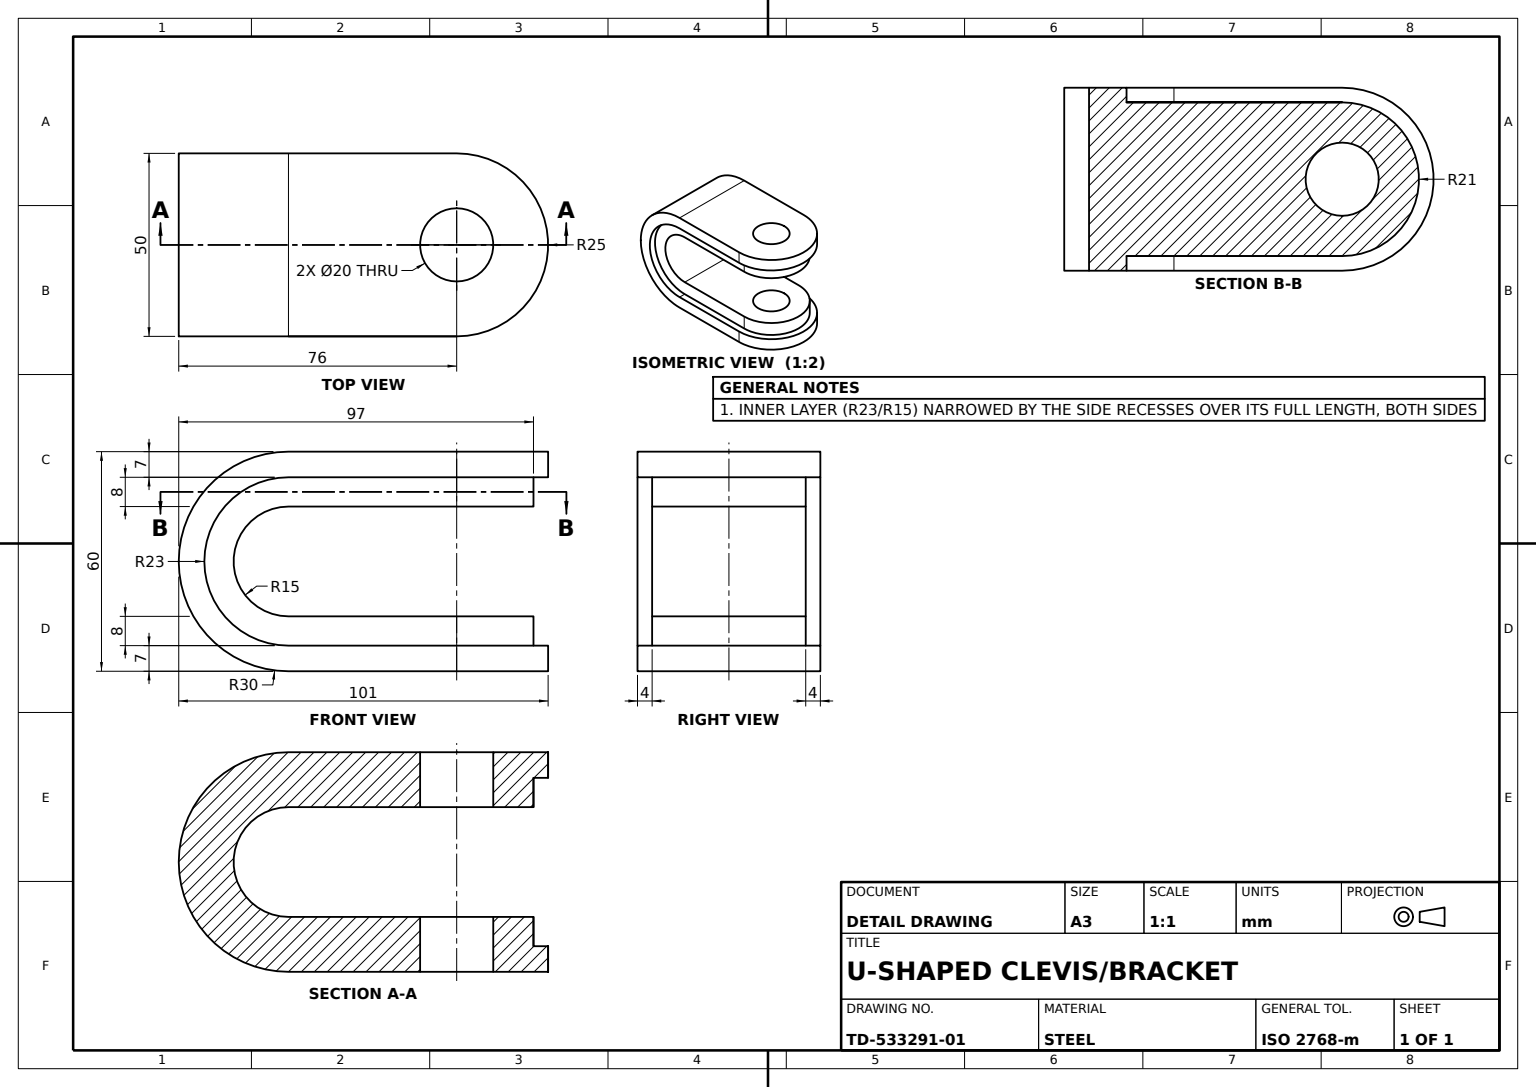
from build123d import *

# Parameters (mm, degrees)
U_FORK_BASE_DEPTH   = 50
U_START             = -50
U_WRAP_LAYER_DEPTH  = 50
WRAP_START          = -4
WRAP_RECESS_1_DEPTH = 4
WRAP_RECESS_2_DEPTH = 4
ARM_PAD_1_DEPTH     = 8
ARM_PAD_2_DEPTH     = 8
ARM_START           = -8
ARM_PAD_3_DEPTH     = 8
ARM_PAD_4_DEPTH     = 8
ARM_PAD_5_DEPTH     = 8
PIN_HOLE_SKETCH_R   = 10
PIN_HOLE_DEPTH      = 70
FACE_RELIEF_1_DEPTH = 1
FACE_START          = -1
FACE_RELIEF_2_DEPTH = 1


with BuildPart() as part:
    # U Fork Profile Sketch → U Fork Base (new body)
    with BuildSketch(Plane.XY):
        with BuildLine():
            ThreePointArc((0, 53), (-23, 30), (0, 7))
            Line((0, 7), (46, 7))
            Line((46, 7), (46, 0))
            Line((46, 0), (0, 0))
            ThreePointArc((0, 0), (-30, 30), (0, 60))
            Line((0, 60), (46, 60))
            Line((46, 60), (46, 53))
            Line((46, 53), (0, 53))
        make_face()
    extrude(amount=U_FORK_BASE_DEPTH)

    # U Wrap Layer Sketch → U Wrap Layer (add)
    with BuildSketch(Plane.XY.offset(50).offset(U_START)):
        with BuildLine():
            Line((0, 53), (46, 53))
            Line((46, 53), (46, 45))
            Line((46, 45), (0, 45))
            ThreePointArc((0, 45), (-15, 30), (0, 15))
            Line((0, 15), (46, 15))
            Line((46, 15), (46, 7))
            Line((46, 7), (0, 7))
            ThreePointArc((0, 7), (-23, 30), (0, 53))
        make_face()
    extrude(amount=U_WRAP_LAYER_DEPTH)

    # Wrap Recess 1 Sketch → Wrap Recess 1 (cut)
    with BuildSketch(Plane.XY.offset(50).offset(WRAP_START)):
        with BuildLine():
            Line((0, 45), (46, 45))
            Line((46, 45), (46, 53))
            Line((46, 53), (0, 53))
            ThreePointArc((0, 53), (-23, 30), (0, 7))
            Line((0, 7), (46, 7))
            Line((46, 7), (46, 15))
            Line((46, 15), (0, 15))
            ThreePointArc((0, 15), (-15, 30), (0, 45))
        make_face()
    extrude(amount=WRAP_RECESS_1_DEPTH, mode=Mode.SUBTRACT)

    # Wrap Recess 2 Sketch → Wrap Recess 2 (cut)
    with BuildSketch(Plane(origin=(0, 0, 0), x_dir=(-1, 0, 0), z_dir=(0, 0, -1))):
        with BuildLine():
            Line((-46, 45), (0, 45))
            ThreePointArc((0, 45), (15, 30), (0, 15))
            Line((0, 15), (-46, 15))
            Line((-46, 15), (-46, 7))
            Line((-46, 7), (0, 7))
            ThreePointArc((0, 7), (23, 30), (0, 53))
            Line((0, 53), (-46, 53))
            Line((-46, 53), (-46, 45))
        make_face()
    extrude(amount=-WRAP_RECESS_2_DEPTH, mode=Mode.SUBTRACT)

    # Arm Pad 1 Sketch → Arm Pad 1 (add)
    with BuildSketch(Plane.XZ.offset(-45)):
        with BuildLine():
            ThreePointArc((46, 10), (61, 25), (46, 40))
            Line((46, 40), (46, 10))
        make_face()
    extrude(amount=-ARM_PAD_1_DEPTH)

    # Arm Pad 2 Sketch → Arm Pad 2 (add)
    with BuildSketch(Plane.XZ.offset(-45)):
        with BuildLine():
            Line((46, 46), (46, 40))
            ThreePointArc((46, 40), (61, 25), (46, 10))
            Line((46, 10), (46, 4))
            ThreePointArc((46, 4), (67, 25), (46, 46))
        make_face()
    extrude(amount=-ARM_PAD_2_DEPTH)

    # Arm Pad 3 Sketch → Arm Pad 3 (add)
    with BuildSketch(Plane(origin=(0, 15, 0), x_dir=(1, 0, 0), z_dir=(0, 1, 0)).offset(ARM_START)):
        with BuildLine():
            ThreePointArc((46, -40), (61, -25), (46, -10))
            Line((46, -10), (46, -40))
        make_face()
        with BuildLine():
            ThreePointArc((46, -46), (67, -25), (46, -4))
            Line((46, -4), (46, -10))
            ThreePointArc((46, -10), (61, -25), (46, -40))
            Line((46, -40), (46, -46))
        make_face()
    extrude(amount=ARM_PAD_3_DEPTH)

    # Arm Pad 4 Sketch → Arm Pad 4 (add)
    with BuildSketch(Plane(origin=(0, 60, 0), x_dir=(1, 0, 0), z_dir=(0, 1, 0)).offset(ARM_START)):
        with BuildLine():
            ThreePointArc((46, -50), (71, -25), (46, 0))
            Line((46, 0), (46, -4))
            ThreePointArc((46, -4), (67, -25), (46, -46))
            Line((46, -46), (46, -50))
        make_face()
        with BuildLine():
            ThreePointArc((46, -46), (67, -25), (46, -4))
            Line((46, -4), (46, -46))
        make_face()
    extrude(amount=ARM_PAD_4_DEPTH)

    # Arm Pad 5 Sketch → Arm Pad 5 (add)
    with BuildSketch(Plane.XZ):
        with BuildLine():
            Line((46, 50), (46, 0))
            ThreePointArc((46, 0), (71, 25), (46, 50))
        make_face()
    extrude(amount=-ARM_PAD_5_DEPTH)

    # Pin Hole Sketch → Pin Hole (cut)
    with BuildSketch(Plane.XZ):
        with Locations(Location((46, 25, 0), (0, 0, 270))):
            Circle(PIN_HOLE_SKETCH_R)
    extrude(amount=-PIN_HOLE_DEPTH, mode=Mode.SUBTRACT)

    # Face Relief 1 Sketch → Face Relief 1 (cut)
    with BuildSketch(Plane.XZ.offset(-52)):
        with BuildLine():
            Line((46, 50), (46, 46))
            ThreePointArc((46, 46), (67, 25), (46, 4))
            Line((46, 4), (46, 0))
            ThreePointArc((46, 0), (71, 25), (46, 50))
        make_face()
    extrude(amount=-FACE_RELIEF_1_DEPTH, mode=Mode.SUBTRACT)

    # Face Relief 2 Sketch → Face Relief 2 (cut)
    with BuildSketch(Plane(origin=(0, 8, 0), x_dir=(1, 0, 0), z_dir=(0, 1, 0)).offset(FACE_START)):
        with BuildLine():
            Line((46, 0), (46, -4))
            ThreePointArc((46, -4), (67, -25), (46, -46))
            Line((46, -46), (46, -50))
            ThreePointArc((46, -50), (71, -25), (46, 0))
        make_face()
    extrude(amount=FACE_RELIEF_2_DEPTH, mode=Mode.SUBTRACT)


solid = part.part
